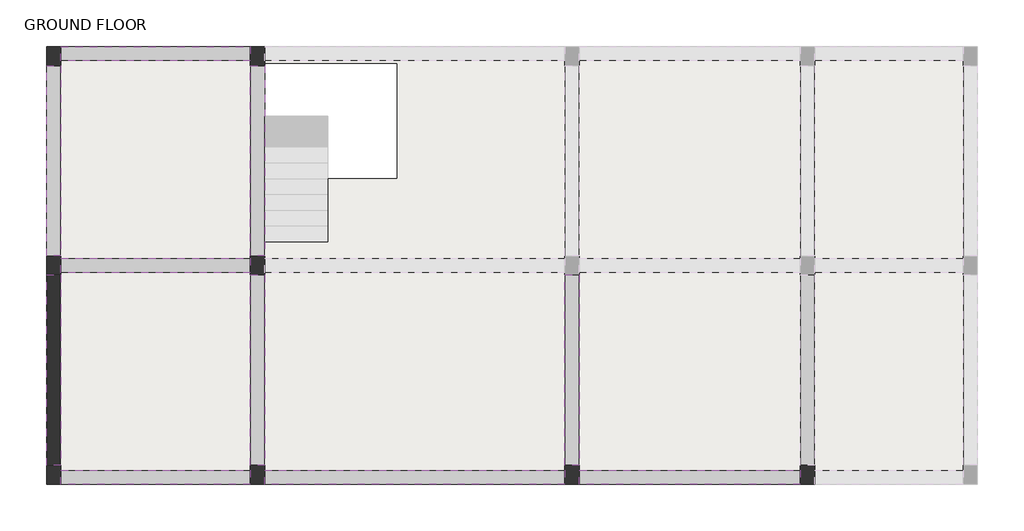
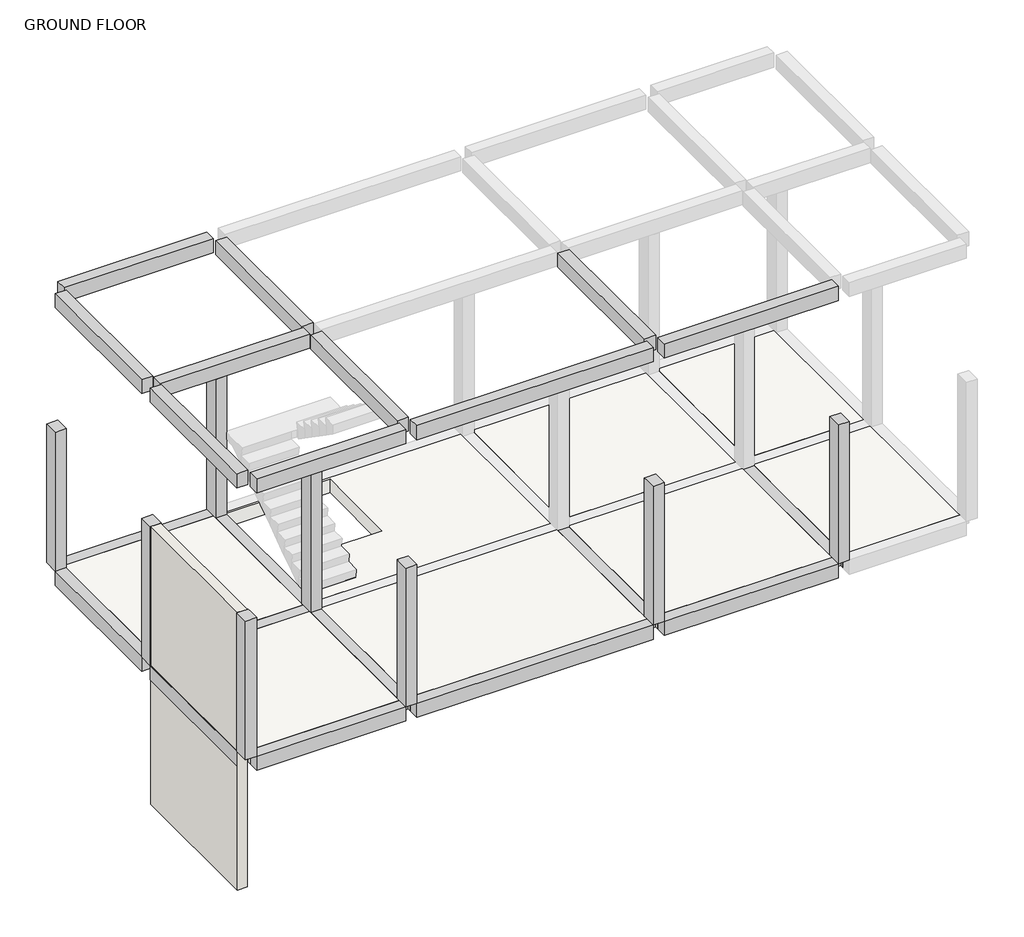
# One storey, part 1 of 2: 21 beams, 8 columns, 4 walls, 2 slabs.
"""IFC4 building model written with IfcOpenShell, lengths in millimetres."""

from ifc_helpers import new_model, si_unit, frame, origin, place, context, project, spatial, polyline, outline, extrude, faceted_brep, element, save

model = new_model("IFC4")

# Units and contexts
model_context = context("Model", 3, world=origin())
ifc_project = project(units=[si_unit("LENGTHUNIT", "METRE", prefix="MILLI")], contexts=[model_context])

# Site, building, storey
site = spatial("IfcSite", under=ifc_project)
building = spatial("IfcBuilding", under=site)
storey = spatial("IfcBuildingStorey", under=building, Name="GROUND FLOOR", Elevation=0.0)

# Beams
placement = place(None, origin())
element("IfcBeam", 1, ObjectType="M_Concrete-Rectangular Beam : 100MM X 200MM", at=placement, inside=storey, context=model_context, shape_type="SweptSolid", body=[
    extrude(outline(polyline([(-5114.1068817, 5712.0180792), (-5342.7068817, 5712.0180792), (-5342.7068817, 8772.8765586), (-5114.1068817, 8772.8765586), (-5114.1068817, 5712.0180792)])), frame((0.0, 0.0, -304.8), z_axis=(0.0, 0.0, 1.0), x_axis=(1.0, 0.0, 0.0)), (0.0, 0.0, 1.0), 304.8),
])
element("IfcBeam", 2, ObjectType="M_Concrete-Rectangular Beam : 100MM X 200MM", at=placement, inside=storey, context=model_context, shape_type="Brep", body=[
    faceted_brep([(-2066.1068817, 2041.8765586, 0.0), (-2066.1068817, 2270.4765586, 0.0), (-5114.1068817, 2270.4765586, 0.0), (-5114.1068817, 2041.8765586, 0.0), (-2066.1068817, 2041.8765586, -304.8), (-5114.1068817, 2041.8765586, -304.8), (-2066.1068817, 2270.4765586, -304.8), (-5114.1068817, 2270.4765586, -304.8), (-2066.1068817, 2270.4765586, -300.0), (-5114.1068817, 2270.4765586, -300.0)], [[[0, 1, 2, 3]], [[4, 0, 3, 5]], [[6, 4, 5, 7]], [[1, 8, 6, 7, 9, 2]], [[1, 0, 4, 6, 8]], [[3, 2, 9, 7, 5]]]),
])
element("IfcBeam", 3, ObjectType="M_Concrete-Rectangular Beam : 100MM X 200MM", at=placement, inside=storey, context=model_context, shape_type="SweptSolid", body=[
    extrude(outline(polyline([(-5114.1068817, 2346.6765586), (-5342.7068817, 2346.6765586), (-5342.7068817, 5407.2180792), (-5114.1068817, 5407.2180792), (-5114.1068817, 2346.6765586)])), frame((0.0, 0.0, -304.8), z_axis=(0.0, 0.0, 1.0), x_axis=(1.0, 0.0, 0.0)), (0.0, 0.0, 1.0), 304.8),
])
element("IfcBeam", 4, ObjectType="M_Concrete-Rectangular Beam : 100MM X 200MM", at=placement, inside=storey, context=model_context, shape_type="Brep", body=[
    faceted_brep([(2988.1931183, 2041.8765586, 0.0), (2988.1931183, 2270.4765586, 0.0), (-1837.5068817, 2270.4765586, 0.0), (-1837.5068817, 2041.8765586, 0.0), (2988.1931183, 2041.8765586, -304.8), (-1837.5068817, 2041.8765586, -304.8), (2988.1931183, 2270.4765586, -304.8), (-1837.5068817, 2270.4765586, -304.8), (-1837.5068817, 2270.4765586, -300.0)], [[[0, 1, 2, 3]], [[4, 0, 3, 5]], [[6, 4, 5, 7]], [[1, 6, 7, 8, 2]], [[1, 0, 4, 6]], [[3, 2, 8, 7, 5]]]),
])
element("IfcBeam", 5, ObjectType="M_Concrete-Rectangular Beam : 100MM X 200MM", at=placement, inside=storey, context=model_context, shape_type="Brep", body=[
    faceted_brep([(6773.0931183, 2041.8765586, 0.0), (6773.0931183, 2270.4765586, 0.0), (3217.0931183, 2270.4765586, 0.0), (3217.0931183, 2041.8765586, 0.0), (6773.0931183, 2041.8765586, -304.8), (3217.0931183, 2041.8765586, -304.8), (6773.0931183, 2270.4765586, -304.8), (3217.0931183, 2270.4765586, -304.8), (6773.0931183, 2270.4765586, -300.0), (3217.0931183, 2270.4765586, -300.0)], [[[0, 1, 2, 3]], [[4, 0, 3, 5]], [[6, 4, 5, 7]], [[1, 8, 6, 7, 9, 2]], [[1, 0, 4, 6, 8]], [[3, 2, 9, 7, 5]]]),
])
element("IfcBeam", 6, ObjectType="M_Concrete-Rectangular Beam : 100MM X 200MM", at=placement, inside=storey, context=model_context, shape_type="Brep", body=[
    faceted_brep([(-2066.1068817, 8849.0765586, 0.0), (-2066.1068817, 9077.6765586, 0.0), (-5114.1068817, 9077.6765586, 0.0), (-5114.1068817, 8849.0765586, 0.0), (-2066.1068817, 8849.0765586, -304.8), (-2066.1068817, 8849.0765586, -300.0), (-5114.1068817, 8849.0765586, -300.0), (-5114.1068817, 8849.0765586, -304.8), (-2066.1068817, 9077.6765586, -304.8), (-5114.1068817, 9077.6765586, -304.8)], [[[0, 1, 2, 3]], [[4, 5, 0, 3, 6, 7]], [[8, 4, 7, 9]], [[1, 8, 9, 2]], [[1, 0, 5, 4, 8]], [[3, 2, 9, 7, 6]]]),
])
element("IfcBeam", 7, ObjectType="M_Concrete-Rectangular Beam : 100MM X 200MM", at=placement, inside=storey, context=model_context, shape_type="Brep", body=[
    faceted_brep([(-2066.1068817, 5445.3180792, 0.0), (-2066.1068817, 5673.9180792, 0.0), (-5114.1068817, 5673.9180792, 0.0), (-5114.1068817, 5445.3180792, 0.0), (-2066.1068817, 5673.9180792, -300.0), (-2066.1068817, 5673.9180792, -304.8), (-5114.1068817, 5673.9180792, -304.8), (-5114.1068817, 5673.9180792, -300.0), (-2066.1068817, 5445.3180792, -304.8), (-5114.1068817, 5445.3180792, -304.8), (-2066.1068817, 5445.3180792, -300.0), (-5114.1068817, 5445.3180792, -300.0)], [[[0, 1, 2, 3]], [[2, 1, 4, 5, 6, 7]], [[5, 8, 9, 6]], [[8, 10, 0, 3, 11, 9]], [[1, 0, 10, 8, 5, 4]], [[3, 2, 7, 6, 9, 11]]]),
])
element("IfcBeam", 8, ObjectType="M_Concrete-Rectangular Beam : 100MM X 200MM", at=placement, inside=storey, context=model_context, shape_type="Brep", body=[
    faceted_brep([(7001.6931183, 5407.2180792, 0.0), (6773.0931183, 5407.2180792, 0.0), (6773.0931183, 2346.6765586, 0.0), (7001.6931183, 2346.6765586, 0.0), (7001.6931183, 2346.6765586, -300.0), (7001.6931183, 2346.6765586, -304.8), (7001.6931183, 5407.2180792, -304.8), (7001.6931183, 5407.2180792, -300.0), (6773.0931183, 5407.2180792, -304.8), (6773.0931183, 2346.6765586, -304.8), (6773.0931183, 5407.2180792, -300.0), (6773.0931183, 2346.6765586, -300.0)], [[[0, 1, 2, 3]], [[0, 3, 4, 5, 6, 7]], [[8, 6, 5, 9]], [[2, 1, 10, 8, 9, 11]], [[1, 0, 7, 6, 8, 10]], [[3, 2, 11, 9, 5, 4]]]),
])
element("IfcBeam", 9, ObjectType="M_Concrete-Rectangular Beam : 100MM X 200MM", at=placement, inside=storey, context=model_context, shape_type="Brep", body=[
    faceted_brep([(3217.0931183, 5407.2180792, 0.0), (2988.4931183, 5407.2180792, 0.0), (2988.4931183, 2346.6765586, 0.0), (3217.0931183, 2346.6765586, 0.0), (3217.0931183, 2346.6765586, -300.0), (3217.0931183, 2346.6765586, -304.8), (3217.0931183, 5407.2180792, -304.8), (3217.0931183, 5407.2180792, -300.0), (2988.4931183, 5407.2180792, -304.8), (2988.4931183, 2346.6765586, -304.8), (2988.4931183, 5407.2180792, -300.0), (2988.4931183, 2346.6765586, -300.0)], [[[0, 1, 2, 3]], [[0, 3, 4, 5, 6, 7]], [[8, 6, 5, 9]], [[2, 1, 10, 8, 9, 11]], [[1, 0, 7, 6, 8, 10]], [[3, 2, 11, 9, 5, 4]]]),
])
element("IfcBeam", 10, ObjectType="M_Concrete-Rectangular Beam : 100MM X 200MM", at=placement, inside=storey, context=model_context, shape_type="Brep", body=[
    faceted_brep([(-1837.5068817, 5407.2180792, 0.0), (-2066.1068817, 5407.2180792, 0.0), (-2066.1068817, 2346.6765586, 0.0), (-1837.5068817, 2346.6765586, 0.0), (-1837.5068817, 2346.6765586, -300.0), (-1837.5068817, 2346.6765586, -304.8), (-1837.5068817, 5407.2180792, -304.8), (-1837.5068817, 5407.2180792, -300.0), (-2066.1068817, 5407.2180792, -304.8), (-2066.1068817, 2346.6765586, -304.8)], [[[0, 1, 2, 3]], [[0, 3, 4, 5, 6, 7]], [[8, 6, 5, 9]], [[1, 8, 9, 2]], [[1, 0, 7, 6, 8]], [[3, 2, 9, 5, 4]]]),
])
element("IfcBeam", 11, ObjectType="M_Concrete-Rectangular Beam : 100MM X 200MM", at=placement, inside=storey, context=model_context, shape_type="Brep", body=[
    faceted_brep([(-1837.5068817, 8772.8765586, 0.0), (-2066.1068817, 8772.8765586, 0.0), (-2066.1068817, 5712.0180792, 0.0), (-1837.5068817, 5712.0180792, 0.0), (-1837.5068817, 5940.7765586, 0.0), (-1837.5068817, 8772.8765586, -304.8), (-1837.5068817, 5712.0180792, -300.0), (-1837.5068817, 5712.0180792, -304.8), (-2066.1068817, 8772.8765586, -304.8), (-2066.1068817, 5712.0180792, -304.8), (-2066.1068817, 8772.8765586, -300.0), (-2066.1068817, 5712.0180792, -300.0)], [[[0, 1, 2, 3, 4]], [[5, 0, 4, 3, 6, 7]], [[8, 5, 7, 9]], [[2, 1, 10, 8, 9, 11]], [[1, 0, 5, 8, 10]], [[3, 2, 11, 9, 7, 6]]]),
])
element("IfcBeam", 12, ObjectType="M_Concrete-Rectangular Beam : 100MM X 200MM", at=placement, inside=storey, context=model_context, shape_type="SweptSolid", body=[
    extrude(outline(polyline([(-5114.1068817, 5712.0180792), (-5342.7068817, 5712.0180792), (-5342.7068817, 8772.8765586), (-5114.1068817, 8772.8765586), (-5114.1068817, 5712.0180792)])), frame((0.0, 0.0, 5695.2), z_axis=(0.0, 0.0, 1.0), x_axis=(1.0, 0.0, 0.0)), (0.0, 0.0, 1.0), 304.8),
])
element("IfcBeam", 13, ObjectType="M_Concrete-Rectangular Beam : 100MM X 200MM", at=placement, inside=storey, context=model_context, shape_type="Brep", body=[
    faceted_brep([(-2066.1068817, 2041.8765586, 6000.0), (-2066.1068817, 2270.4765586, 6000.0), (-5114.1068817, 2270.4765586, 6000.0), (-5114.1068817, 2041.8765586, 6000.0), (-2066.1068817, 2041.8765586, 5695.2), (-5114.1068817, 2041.8765586, 5695.2), (-2066.1068817, 2270.4765586, 5695.2), (-5114.1068817, 2270.4765586, 5695.2), (-2066.1068817, 2270.4765586, 5700.0), (-5114.1068817, 2270.4765586, 5700.0)], [[[0, 1, 2, 3]], [[4, 0, 3, 5]], [[6, 4, 5, 7]], [[1, 8, 6, 7, 9, 2]], [[1, 0, 4, 6, 8]], [[3, 2, 9, 7, 5]]]),
])
element("IfcBeam", 14, ObjectType="M_Concrete-Rectangular Beam : 100MM X 200MM", at=placement, inside=storey, context=model_context, shape_type="SweptSolid", body=[
    extrude(outline(polyline([(-5114.1068817, 2346.6765586), (-5342.7068817, 2346.6765586), (-5342.7068817, 5407.2180792), (-5114.1068817, 5407.2180792), (-5114.1068817, 2346.6765586)])), frame((0.0, 0.0, 5695.2), z_axis=(0.0, 0.0, 1.0), x_axis=(1.0, 0.0, 0.0)), (0.0, 0.0, 1.0), 304.8),
])
element("IfcBeam", 15, ObjectType="M_Concrete-Rectangular Beam : 100MM X 200MM", at=placement, inside=storey, context=model_context, shape_type="Brep", body=[
    faceted_brep([(2988.1931183, 2041.8765586, 6000.0), (2988.1931183, 2270.4765586, 6000.0), (-1837.5068817, 2270.4765586, 6000.0), (-1837.5068817, 2041.8765586, 6000.0), (2988.1931183, 2041.8765586, 5695.2), (-1837.5068817, 2041.8765586, 5695.2), (2988.1931183, 2270.4765586, 5695.2), (-1837.5068817, 2270.4765586, 5695.2), (-1837.5068817, 2270.4765586, 5700.0)], [[[0, 1, 2, 3]], [[4, 0, 3, 5]], [[6, 4, 5, 7]], [[1, 6, 7, 8, 2]], [[1, 0, 4, 6]], [[3, 2, 8, 7, 5]]]),
])
element("IfcBeam", 16, ObjectType="M_Concrete-Rectangular Beam : 100MM X 200MM", at=placement, inside=storey, context=model_context, shape_type="Brep", body=[
    faceted_brep([(6773.0931183, 2041.8765586, 6000.0), (6773.0931183, 2270.4765586, 6000.0), (3217.0931183, 2270.4765586, 6000.0), (3217.0931183, 2041.8765586, 6000.0), (6773.0931183, 2041.8765586, 5695.2), (3217.0931183, 2041.8765586, 5695.2), (6773.0931183, 2270.4765586, 5695.2), (3217.0931183, 2270.4765586, 5695.2), (6773.0931183, 2270.4765586, 5700.0), (3217.0931183, 2270.4765586, 5700.0)], [[[0, 1, 2, 3]], [[4, 0, 3, 5]], [[6, 4, 5, 7]], [[1, 8, 6, 7, 9, 2]], [[1, 0, 4, 6, 8]], [[3, 2, 9, 7, 5]]]),
])
element("IfcBeam", 17, ObjectType="M_Concrete-Rectangular Beam : 100MM X 200MM", at=placement, inside=storey, context=model_context, shape_type="Brep", body=[
    faceted_brep([(-2066.1068817, 8849.0765586, 6000.0), (-2066.1068817, 9077.6765586, 6000.0), (-5114.1068817, 9077.6765586, 6000.0), (-5114.1068817, 8849.0765586, 6000.0), (-2066.1068817, 8849.0765586, 5695.2), (-2066.1068817, 8849.0765586, 5700.0), (-5114.1068817, 8849.0765586, 5700.0), (-5114.1068817, 8849.0765586, 5695.2), (-2066.1068817, 9077.6765586, 5695.2), (-5114.1068817, 9077.6765586, 5695.2)], [[[0, 1, 2, 3]], [[4, 5, 0, 3, 6, 7]], [[8, 4, 7, 9]], [[1, 8, 9, 2]], [[1, 0, 5, 4, 8]], [[3, 2, 9, 7, 6]]]),
])
element("IfcBeam", 18, ObjectType="M_Concrete-Rectangular Beam : 100MM X 200MM", at=placement, inside=storey, context=model_context, shape_type="Brep", body=[
    faceted_brep([(-2066.1068817, 5673.9180792, 6000.0), (-5114.1068817, 5673.9180792, 6000.0), (-5114.1068817, 5445.3180792, 6000.0), (-2066.1068817, 5445.3180792, 6000.0), (-2066.1068817, 5673.9180792, 5700.0), (-2066.1068817, 5673.9180792, 5695.2), (-5114.1068817, 5673.9180792, 5695.2), (-5114.1068817, 5673.9180792, 5700.0), (-2066.1068817, 5445.3180792, 5695.2), (-5114.1068817, 5445.3180792, 5695.2), (-2066.1068817, 5445.3180792, 5700.0), (-5114.1068817, 5445.3180792, 5700.0)], [[[0, 1, 2, 3]], [[1, 0, 4, 5, 6, 7]], [[5, 8, 9, 6]], [[8, 10, 3, 2, 11, 9]], [[0, 3, 10, 8, 5, 4]], [[2, 1, 7, 6, 9, 11]]]),
])
element("IfcBeam", 19, ObjectType="M_Concrete-Rectangular Beam : 100MM X 200MM", at=placement, inside=storey, context=model_context, shape_type="SweptSolid", body=[
    extrude(outline(polyline([(2988.4931183, 5407.2180792), (3217.0931183, 5407.2180792), (3217.0931183, 2346.6765586), (2988.4931183, 2346.6765586), (2988.4931183, 5407.2180792)])), frame((0.0, 0.0, 5695.2), z_axis=(0.0, 0.0, 1.0), x_axis=(1.0, 0.0, 0.0)), (0.0, 0.0, 1.0), 304.8),
])
element("IfcBeam", 20, ObjectType="M_Concrete-Rectangular Beam : 100MM X 200MM", at=placement, inside=storey, context=model_context, shape_type="SweptSolid", body=[
    extrude(outline(polyline([(-2066.1068817, 5407.2180792), (-1837.5068817, 5407.2180792), (-1837.5068817, 2346.6765586), (-2066.1068817, 2346.6765586), (-2066.1068817, 5407.2180792)])), frame((0.0, 0.0, 5695.2), z_axis=(0.0, 0.0, 1.0), x_axis=(1.0, 0.0, 0.0)), (0.0, 0.0, 1.0), 304.8),
])
element("IfcBeam", 21, ObjectType="M_Concrete-Rectangular Beam : 100MM X 200MM", at=placement, inside=storey, context=model_context, shape_type="Brep", body=[
    faceted_brep([(-1837.5068817, 8772.8765586, 6000.0), (-2066.1068817, 8772.8765586, 6000.0), (-2066.1068817, 5712.0180792, 6000.0), (-1837.5068817, 5712.0180792, 6000.0), (-1837.5068817, 5940.7765586, 6000.0), (-1837.5068817, 8772.8765586, 5695.2), (-1837.5068817, 5712.0180792, 5695.2), (-2066.1068817, 8772.8765586, 5695.2), (-2066.1068817, 5712.0180792, 5695.2)], [[[0, 1, 2, 3, 4]], [[5, 0, 4, 3, 6]], [[7, 5, 6, 8]], [[1, 7, 8, 2]], [[1, 0, 5, 7]], [[3, 2, 8, 6]]]),
])

# Columns
element("IfcColumn", 22, ObjectType="M_Concrete-Rectangular-Column : 9\" X 1' COLUMNS", at=placement, inside=storey, context=model_context, shape_type="Brep", body=[
    faceted_brep([(7001.6931183, 2346.6765586, 0.0), (7001.6931183, 2041.8765586, 0.0), (6773.0931183, 2041.8765586, 0.0), (6773.0931183, 2346.6765586, 0.0), (7001.6931183, 2346.6765586, 2700.0), (7001.6931183, 2346.6765586, 3000.0), (7001.6931183, 2270.4765586, 3000.0), (7001.6931183, 2041.8765586, 3000.0), (6773.0931183, 2041.8765586, 3000.0), (6773.0931183, 2270.4765586, 3000.0), (6773.0931183, 2346.6765586, 3000.0), (6773.0931183, 2346.6765586, 2700.0)], [[[0, 1, 2, 3]], [[1, 0, 4, 5, 6, 7]], [[2, 1, 7, 8]], [[3, 2, 8, 9, 10, 11]], [[0, 3, 11, 10, 5, 4]], [[8, 7, 6, 5, 10, 9]]]),
])
element("IfcColumn", 23, ObjectType="M_Concrete-Rectangular-Column : 9\" X 1' COLUMNS", at=placement, inside=storey, context=model_context, shape_type="Brep", body=[
    faceted_brep([(3217.0931183, 2346.6765586, 0.0), (3217.0931183, 2041.8765586, 0.0), (2988.4931183, 2041.8765586, 0.0), (2988.4931183, 2346.6765586, 0.0), (3217.0931183, 2346.6765586, 2700.0), (3217.0931183, 2346.6765586, 3000.0), (3217.0931183, 2270.4765586, 3000.0), (3217.0931183, 2041.8765586, 3000.0), (2988.4931183, 2041.8765586, 3000.0), (2988.4931183, 2270.4765586, 3000.0), (2988.4931183, 2346.6765586, 3000.0), (2988.4931183, 2346.6765586, 2700.0)], [[[0, 1, 2, 3]], [[1, 0, 4, 5, 6, 7]], [[2, 1, 7, 8]], [[3, 2, 8, 9, 10, 11]], [[0, 3, 11, 10, 5, 4]], [[8, 7, 6, 5, 10, 9]]]),
])
element("IfcColumn", 24, ObjectType="M_Concrete-Rectangular-Column : 9\" X 1' COLUMNS", at=placement, inside=storey, context=model_context, shape_type="Brep", body=[
    faceted_brep([(-1837.5068817, 9077.6765586, 0.0), (-1837.5068817, 8772.8765586, 0.0), (-2066.1068817, 8772.8765586, 0.0), (-2066.1068817, 9077.6765586, 0.0), (-1837.5068817, 9077.6765586, 3000.0), (-1837.5068817, 8849.0765586, 3000.0), (-1837.5068817, 8810.9765586, 3000.0), (-1837.5068817, 8772.8765586, 3000.0), (-2066.1068817, 8772.8765586, 3000.0), (-2066.1068817, 8772.8765586, 2700.0), (-2066.1068817, 8849.0765586, 3000.0), (-2066.1068817, 9077.6765586, 3000.0)], [[[0, 1, 2, 3]], [[1, 0, 4, 5, 6, 7]], [[2, 1, 7, 8, 9]], [[3, 2, 9, 8, 10, 11]], [[0, 3, 11, 4]], [[8, 7, 6, 5, 4, 11, 10]]]),
])
element("IfcColumn", 25, ObjectType="M_Concrete-Rectangular-Column : 9\" X 1' COLUMNS", at=placement, inside=storey, context=model_context, shape_type="Brep", body=[
    faceted_brep([(-1837.5068817, 5712.0180792, 0.0), (-1837.5068817, 5407.2180792, 0.0), (-2066.1068817, 5407.2180792, 0.0), (-2066.1068817, 5712.0180792, 0.0), (-1837.5068817, 5712.0180792, 2700.0), (-1837.5068817, 5712.0180792, 3000.0), (-1837.5068817, 5673.9180792, 3000.0), (-1837.5068817, 5445.3180792, 3000.0), (-1837.5068817, 5407.2180792, 3000.0), (-1837.5068817, 5407.2180792, 2700.0), (-2066.1068817, 5407.2180792, 3000.0), (-2066.1068817, 5445.3180792, 3000.0), (-2066.1068817, 5673.9180792, 3000.0), (-2066.1068817, 5712.0180792, 3000.0), (-2066.1068817, 5712.0180792, 2700.0)], [[[0, 1, 2, 3]], [[1, 0, 4, 5, 6, 7, 8, 9]], [[2, 1, 9, 8, 10]], [[3, 2, 10, 11, 12, 13, 14]], [[0, 3, 14, 13, 5, 4]], [[10, 8, 7, 6, 5, 13, 12, 11]]]),
])
element("IfcColumn", 26, ObjectType="M_Concrete-Rectangular-Column : 9\" X 1' COLUMNS", at=placement, inside=storey, context=model_context, shape_type="Brep", body=[
    faceted_brep([(-1837.5068817, 2346.6765586, 0.0), (-1837.5068817, 2041.8765586, 0.0), (-2066.1068817, 2041.8765586, 0.0), (-2066.1068817, 2346.6765586, 0.0), (-1837.5068817, 2346.6765586, 2700.0), (-1837.5068817, 2346.6765586, 3000.0), (-1837.5068817, 2270.4765586, 3000.0), (-1837.5068817, 2041.8765586, 3000.0), (-2066.1068817, 2041.8765586, 3000.0), (-2066.1068817, 2270.4765586, 3000.0), (-2066.1068817, 2346.6765586, 3000.0)], [[[0, 1, 2, 3]], [[1, 0, 4, 5, 6, 7]], [[2, 1, 7, 8]], [[3, 2, 8, 9, 10]], [[0, 3, 10, 5, 4]], [[8, 7, 6, 5, 10, 9]]]),
])
element("IfcColumn", 27, ObjectType="M_Concrete-Rectangular-Column : 9\" X 1' COLUMNS", at=placement, inside=storey, context=model_context, shape_type="Brep", body=[
    faceted_brep([(-5114.1068817, 2346.6765586, 0.0), (-5114.1068817, 2041.8765586, 0.0), (-5342.7068817, 2041.8765586, 0.0), (-5342.7068817, 2346.6765586, 0.0), (-5114.1068817, 2346.6765586, 3000.0), (-5114.1068817, 2270.4765586, 3000.0), (-5114.1068817, 2041.8765586, 3000.0), (-5342.7068817, 2041.8765586, 3000.0), (-5342.7068817, 2346.6765586, 3000.0)], [[[0, 1, 2, 3]], [[4, 5, 6, 1, 0]], [[6, 7, 2, 1]], [[7, 8, 3, 2]], [[8, 4, 0, 3]], [[4, 8, 7, 6, 5]]]),
])
element("IfcColumn", 28, ObjectType="M_Concrete-Rectangular-Column : 9\" X 1' COLUMNS", at=placement, inside=storey, context=model_context, shape_type="Brep", body=[
    faceted_brep([(-5114.1068817, 5712.0180792, 0.0), (-5114.1068817, 5407.2180792, 0.0), (-5342.7068817, 5407.2180792, 0.0), (-5342.7068817, 5712.0180792, 0.0), (-5114.1068817, 5712.0180792, 3000.0), (-5114.1068817, 5673.9180792, 3000.0), (-5114.1068817, 5445.3180792, 3000.0), (-5114.1068817, 5407.2180792, 3000.0), (-5342.7068817, 5407.2180792, 3000.0), (-5342.7068817, 5712.0180792, 3000.0)], [[[0, 1, 2, 3]], [[4, 5, 6, 7, 1, 0]], [[7, 8, 2, 1]], [[8, 9, 3, 2]], [[9, 4, 0, 3]], [[4, 9, 8, 7, 6, 5]]]),
])
element("IfcColumn", 29, ObjectType="M_Concrete-Rectangular-Column : 9\" X 1' COLUMNS", at=placement, inside=storey, context=model_context, shape_type="Brep", body=[
    faceted_brep([(-5114.1068817, 9077.6765586, 0.0), (-5114.1068817, 8772.8765586, 0.0), (-5342.7068817, 8772.8765586, 0.0), (-5342.7068817, 9077.6765586, 0.0), (-5114.1068817, 9077.6765586, 3000.0), (-5114.1068817, 8849.0765586, 3000.0), (-5114.1068817, 8772.8765586, 3000.0), (-5342.7068817, 8772.8765586, 3000.0), (-5342.7068817, 9077.6765586, 3000.0)], [[[0, 1, 2, 3]], [[4, 5, 6, 1, 0]], [[6, 7, 2, 1]], [[7, 8, 3, 2]], [[8, 4, 0, 3]], [[4, 8, 7, 6, 5]]]),
])

# Slabs
element("IfcSlab", 30, ObjectType="Generic 300mm", at=placement, inside=storey, context=model_context, shape_type="Brep", body=[
    faceted_brep([(-2066.1068817, 2270.4765586, -300.0), (-5114.1068817, 2270.4765586, -300.0), (-5114.1068817, 5445.3180792, -300.0), (-2066.1068817, 5445.3180792, -300.0), (-2066.1068817, 2270.4765586, 0.0), (-2066.1068817, 2346.6765586, 0.0), (-2066.1068817, 5407.2180792, 0.0), (-2066.1068817, 5445.3180792, 0.0), (-5114.1068817, 5445.3180792, 0.0), (-5114.1068817, 5407.2180792, 0.0), (-5114.1068817, 2346.6765586, 0.0), (-5114.1068817, 2270.4765586, 0.0)], [[[0, 1, 2, 3]], [[4, 5, 6, 7, 8, 9, 10, 11]], [[1, 0, 4, 11]], [[2, 1, 11, 10, 9, 8]], [[3, 2, 8, 7]], [[0, 3, 7, 6, 5, 4]]]),
])
element("IfcSlab", 31, ObjectType="Generic 300mm", at=placement, inside=storey, context=model_context, shape_type="Brep", body=[
    faceted_brep([(2988.4931183, 2270.4765586, -300.0), (-1837.5068817, 2270.4765586, -300.0), (-1837.5068817, 5445.3180792, -300.0), (2988.4931183, 5445.3180792, -300.0), (-1837.5068817, 2270.4765586, 0.0), (2988.1931183, 2270.4765586, 0.0), (2988.4931183, 2270.4765586, 0.0), (2988.4931183, 2346.6765586, 0.0), (2988.4931183, 5407.2180792, 0.0), (2988.4931183, 5445.3180792, 0.0), (-1837.5068817, 5445.3180792, 0.0), (-1837.5068817, 5407.2180792, 0.0), (-1837.5068817, 2346.6765586, 0.0)], [[[0, 1, 2, 3]], [[4, 5, 6, 7, 8, 9, 10, 11, 12]], [[1, 0, 6, 5, 4]], [[2, 1, 4, 12, 11, 10]], [[3, 2, 10, 9]], [[0, 3, 9, 8, 7, 6]]]),
    faceted_brep([(6773.0931183, 2270.4765586, -300.0), (3217.0931183, 2270.4765586, -300.0), (3217.0931183, 5445.3180792, -300.0), (6773.0931183, 5445.3180792, -300.0), (3217.0931183, 2270.4765586, 0.0), (6773.0931183, 2270.4765586, 0.0), (6773.0931183, 2346.6765586, 0.0), (6773.0931183, 5407.2180792, 0.0), (6773.0931183, 5445.3180792, 0.0), (3217.0931183, 5445.3180792, 0.0), (3217.0931183, 5407.2180792, 0.0), (3217.0931183, 2346.6765586, 0.0)], [[[0, 1, 2, 3]], [[4, 5, 6, 7, 8, 9, 10, 11]], [[1, 0, 5, 4]], [[2, 1, 4, 11, 10, 9]], [[3, 2, 9, 8]], [[0, 3, 8, 7, 6, 5]]]),
    faceted_brep([(9389.2931183, 2270.4765586, -300.0), (7001.6931183, 2270.4765586, -300.0), (7001.6931183, 5445.3180792, -300.0), (9389.2931183, 5445.3180792, -300.0), (7001.6931183, 2270.4765586, 0.0), (9387.3931183, 2270.4765586, 0.0), (9389.2931183, 2270.4765586, 0.0), (9389.2931183, 2346.6765586, 0.0), (9389.2931183, 2354.2765586, 0.0), (9389.2931183, 5407.2180792, 0.0), (9389.2931183, 5445.3180792, 0.0), (7001.6931183, 5445.3180792, 0.0), (7001.6931183, 5407.2180792, 0.0), (7001.6931183, 2346.6765586, 0.0)], [[[0, 1, 2, 3]], [[4, 5, 6, 7, 8, 9, 10, 11, 12, 13]], [[1, 0, 6, 5, 4]], [[2, 1, 4, 13, 12, 11]], [[3, 2, 11, 10]], [[0, 3, 10, 9, 8, 7, 6]]]),
    faceted_brep([(7001.6931183, 5673.9180792, -300.0), (7001.6931183, 8849.0765586, -300.0), (9389.2931183, 8849.0765586, -300.0), (9389.2931183, 5673.9180792, -300.0), (7001.6931183, 8849.0765586, 0.0), (7001.6931183, 8772.8765586, 0.0), (7001.6931183, 5712.0180792, 0.0), (7001.6931183, 5673.9180792, 0.0), (9389.2931183, 5673.9180792, 0.0), (9389.2931183, 5712.0180792, 0.0), (9389.2931183, 8772.8765586, 0.0), (9389.2931183, 8849.0765586, 0.0), (9387.3931183, 8849.0765586, 0.0)], [[[0, 1, 2, 3]], [[4, 5, 6, 7, 8, 9, 10, 11, 12]], [[1, 0, 7, 6, 5, 4]], [[2, 1, 4, 12, 11]], [[3, 2, 11, 10, 9, 8]], [[0, 3, 8, 7]]]),
    faceted_brep([(3217.0931183, 5673.9180792, -300.0), (3217.0931183, 8849.0765586, -300.0), (6773.0931183, 8849.0765586, -300.0), (6773.0931183, 5673.9180792, -300.0), (3217.0931183, 8849.0765586, 0.0), (3217.0931183, 8772.8765586, 0.0), (3217.0931183, 5719.6180792, 0.0), (3217.0931183, 5712.0180792, 0.0), (3217.0931183, 5673.9180792, 0.0), (6773.0931183, 5673.9180792, 0.0), (6773.0931183, 5712.0180792, 0.0), (6773.0931183, 8772.8765586, 0.0), (6773.0931183, 8849.0765586, 0.0)], [[[0, 1, 2, 3]], [[4, 5, 6, 7, 8, 9, 10, 11, 12]], [[1, 0, 8, 7, 6, 5, 4]], [[2, 1, 4, 12]], [[3, 2, 12, 11, 10, 9]], [[0, 3, 9, 8]]]),
    faceted_brep([(-1837.5068817, 8849.0765586, -300.0), (2988.4931183, 8849.0765586, -300.0), (2988.4931183, 5673.9180792, -300.0), (-1837.5068817, 5673.9180792, -300.0), (-1837.5068817, 5940.7765586, -300.0), (-821.5068817, 5940.7765586, -300.0), (-821.5068817, 6956.7765586, -300.0), (296.0931183, 6956.7765586, -300.0), (296.0931183, 8810.9765586, -300.0), (-1837.5068817, 8810.9765586, -300.0), (2988.4931183, 8849.0765586, 0.0), (-1837.5068817, 8849.0765586, 0.0), (-1837.5068817, 8810.9765586, 0.0), (296.0931183, 8810.9765586, 0.0), (296.0931183, 6956.7765586, 0.0), (-821.5068817, 6956.7765586, 0.0), (-821.5068817, 5940.7765586, 0.0), (-1837.5068817, 5940.7765586, 0.0), (-1837.5068817, 5712.0180792, 0.0), (-1837.5068817, 5673.9180792, 0.0), (2988.4931183, 5673.9180792, 0.0), (2988.4931183, 5712.0180792, 0.0), (2988.4931183, 5719.6180792, 0.0), (2988.4931183, 8772.8765586, 0.0)], [[[0, 1, 2, 3, 4, 5, 6, 7, 8, 9]], [[10, 11, 12, 13, 14, 15, 16, 17, 18, 19, 20, 21, 22, 23]], [[3, 19, 18, 17, 4]], [[11, 0, 9, 12]], [[1, 0, 11, 10]], [[2, 1, 10, 23, 22, 21, 20]], [[3, 2, 20, 19]], [[5, 16, 15, 6]], [[6, 15, 14, 7]], [[7, 14, 13, 8]], [[8, 13, 12, 9]], [[16, 5, 4, 17]]]),
    faceted_brep([(-5114.1068817, 5673.9180792, -300.0), (-5114.1068817, 8849.0765586, -300.0), (-2066.1068817, 8849.0765586, -300.0), (-2066.1068817, 5673.9180792, -300.0), (-5114.1068817, 8849.0765586, 0.0), (-5114.1068817, 8772.8765586, 0.0), (-5114.1068817, 5712.0180792, 0.0), (-5114.1068817, 5673.9180792, 0.0), (-2066.1068817, 5673.9180792, 0.0), (-2066.1068817, 5712.0180792, 0.0), (-2066.1068817, 8772.8765586, 0.0), (-2066.1068817, 8849.0765586, 0.0)], [[[0, 1, 2, 3]], [[4, 5, 6, 7, 8, 9, 10, 11]], [[1, 0, 7, 6, 5, 4]], [[2, 1, 4, 11]], [[3, 2, 11, 10, 9, 8]], [[0, 3, 8, 7]]]),
])

# Walls
element("IfcWall", 32, ObjectType="Generic - 200mm", at=placement, inside=storey, context=model_context, shape_type="SweptSolid", body=[
    extrude(outline(polyline([(-5328.4068817, 2346.6765586), (-5328.4068817, 5407.2180792), (-5128.4068817, 5407.2180792), (-5128.4068817, 2346.6765586), (-5328.4068817, 2346.6765586)])), frame((0.0, 0.0, -3000.0), z_axis=(0.0, 0.0, 1.0), x_axis=(1.0, 0.0, 0.0)), (0.0, 0.0, 1.0), 6000.0),
])
element("IfcWall", 33, ObjectType="Generic - 200mm", at=placement, inside=storey, context=model_context, shape_type="SweptSolid", body=[
    extrude(outline(polyline([(-5328.4068817, 2346.6765586), (-5328.4068817, 5407.2180792), (-5128.4068817, 5407.2180792), (-5128.4068817, 2346.6765586), (-5328.4068817, 2346.6765586)])), frame((0.0, 0.0, -3000.0), z_axis=(0.0, 0.0, 1.0), x_axis=(1.0, 0.0, 0.0)), (0.0, 0.0, 1.0), 6000.0),
])
element("IfcWall", 34, ObjectType="Generic - 200mm", at=placement, inside=storey, context=model_context, shape_type="SweptSolid", body=[
    extrude(outline(polyline([(-5328.4068817, 2346.6765586), (-5328.4068817, 5407.2180792), (-5128.4068817, 5407.2180792), (-5128.4068817, 2346.6765586), (-5328.4068817, 2346.6765586)])), frame((0.0, 0.0, -3000.0), z_axis=(0.0, 0.0, 1.0), x_axis=(1.0, 0.0, 0.0)), (0.0, 0.0, 1.0), 6000.0),
])
element("IfcWall", 35, ObjectType="Generic - 200mm", at=placement, inside=storey, context=model_context, shape_type="SweptSolid", body=[
    extrude(outline(polyline([(-5328.4068817, 2346.6765586), (-5328.4068817, 5407.2180792), (-5128.4068817, 5407.2180792), (-5128.4068817, 2346.6765586), (-5328.4068817, 2346.6765586)])), frame((0.0, 0.0, -304.8), z_axis=(0.0, 0.0, 1.0), x_axis=(1.0, 0.0, 0.0)), (0.0, 0.0, 1.0), 304.8),
])

save(model, "model.ifc")

# Revit data of these elements
# Type "M_Concrete-Rectangular Beam : 100MM X 200MM"
#   Length [instance default] = 1524 mm
#   b = 228.6 mm
#   h = 304.8 mm
#   Structural Material [instance default] = Concrete, Cast-in-Place gray
#   Assembly Code = ""
# Type "M_Concrete-Rectangular-Column : 9\" X 1' COLUMNS"
#   b = 228.6 mm
#   h = 304.8 mm
#   Structural Material [instance default] = Concrete, Cast-in-Place gray
# Type "Generic 300mm"
#   Function = 0
#   Layers, outside or top first: 300 mm no material (function 1)
# Type "Generic - 200mm"
#   Layers, outside or top first: 200 mm no material (function 1)
# Elements 1, 2, 3, 4, 5, 6, 7, 8, 9, 10, 11, 12, 13, 14, 15, 16, 17, 18, 19, 20, 21 (IfcBeam, "M_Concrete-Rectangular Beam : 100MM X 200MM")
#   Structural Material = Concrete, Cast-in-Place gray
#   Phase Created = New Construction
#   Materials on its faces: "Concrete, Cast-in-Place gray"
# Elements 22, 23, 24, 25, 26, 27, 28, 29 (IfcColumn, "M_Concrete-Rectangular-Column : 9\" X 1' COLUMNS")
#   Structural Material = Concrete, Cast-in-Place gray
#   Phase Created = New Construction
#   Materials on its faces: "Concrete, Cast-in-Place gray"
# Elements 30, 31 (IfcSlab, "Generic 300mm")
#   Height Offset From Level = 0 mm
#   built-in parameter 1001954 = 1
#   Phase Created = New Construction
#   Materials on its faces: "Default Floor"
# Elements 32, 33, 34 (IfcWall, "Generic - 200mm")
#   built-in parameter 1001111 = -3000 mm
#   Top Offset = 0 mm
#   Base Offset = -3000 mm
#   wall height = 6000 mm
#   Phase Created = New Construction
#   Base Constraint = GROUND FLOOR
#   Top Constraint = FIRST FLOOR
#   Materials on its faces: "Default Wall"
# Element 35 (IfcWall, "Generic - 200mm")
#   built-in parameter 1001111 = -304.8 mm
#   Top Offset = 0 mm
#   Base Offset = -304.8 mm
#   wall height = 304.8 mm
#   Phase Created = New Construction
#   Base Constraint = GROUND FLOOR
#   Top Constraint = GROUND FLOOR
#   Materials on its faces: "Default Wall"
# Materials
#   "Concrete, Cast-in-Place gray": class "Concrete", colour RGB 192 192 192, transparency 0, Description = "Cast-in-place concrete", Cost = 0
#   "Default Floor": colour RGB 127 127 127, transparency 0, Cost = 0
#   "Default Wall": colour RGB 128 128 128, transparency 0, Cost = 0
